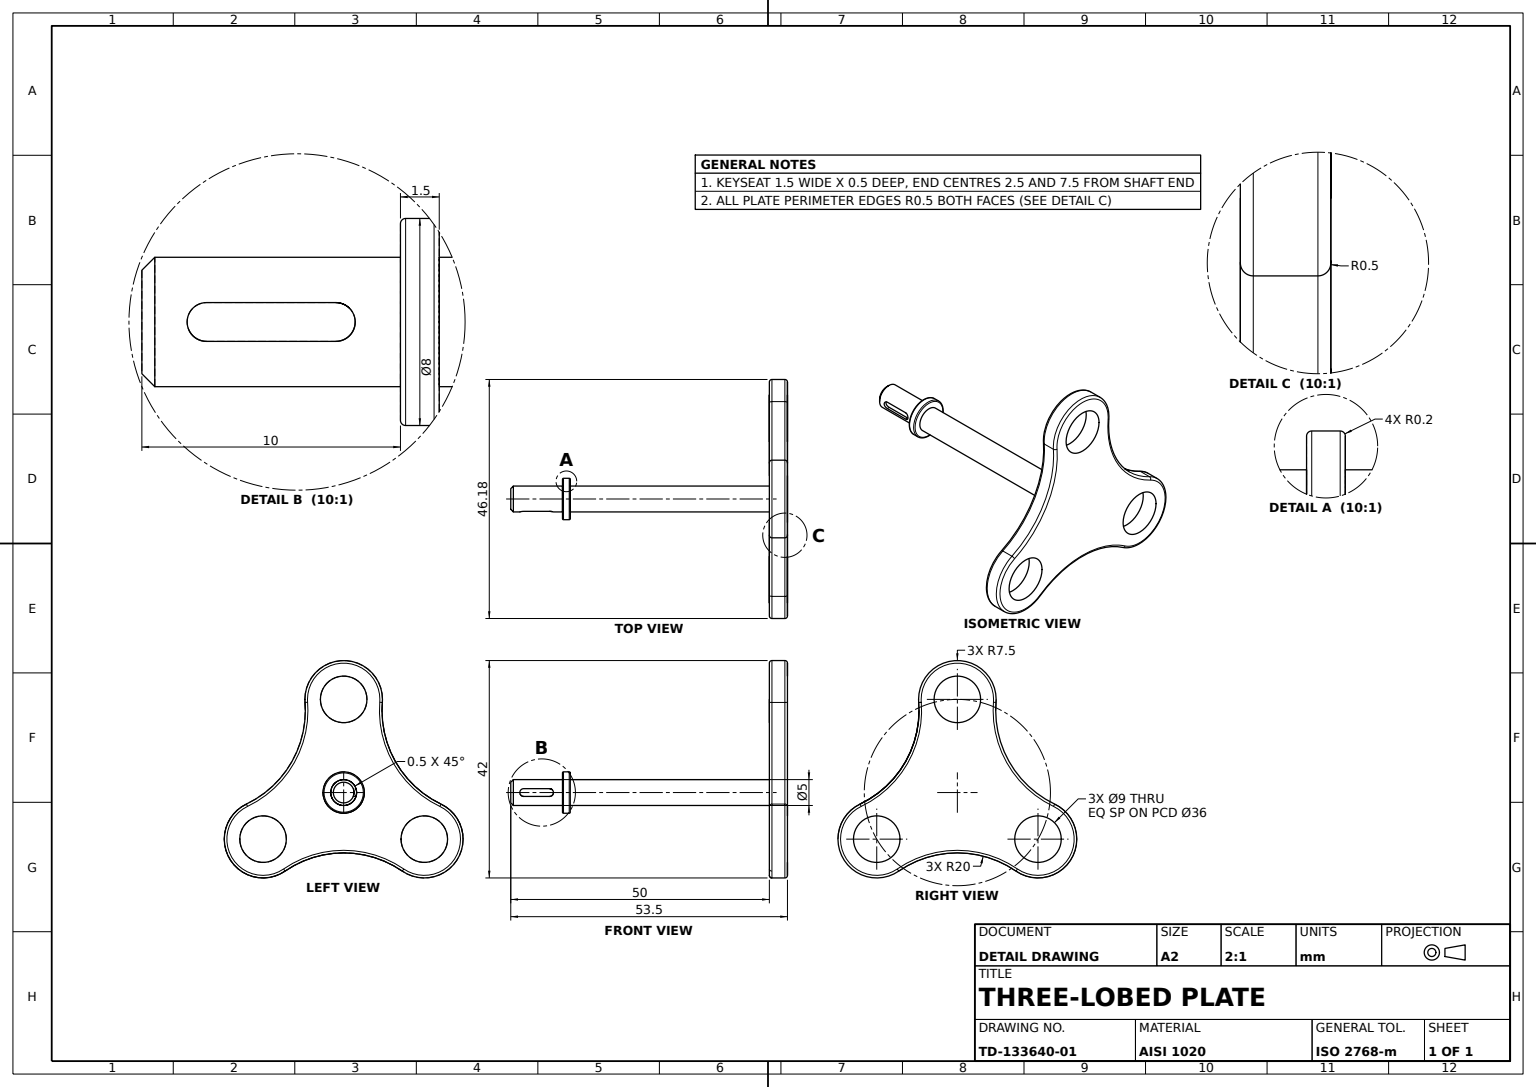
SolidWorks part; units mm, degrees
material "AISI 1020"
ref_plane "Front Plane" through (0, 0, 0) normal (0, 0, 1) x (1, 0, 0)
ref_plane "Top Plane" through (0, 0, 0) normal (0, 1, 0) x (1, 0, 0)
ref_plane "Right Plane" through (0, 0, 0) normal (1, 0, 0) x (0, 0, -1)
sketch "Carrier Plate Profile" plane through (0, 0, 0) normal (0, 0, 1) x (1, 0, 0)
  circle A0 centre (0, 18) radius 7.5
  circle A1 centre (0, 18) radius 4.5
  circle A2 centre (15.5885, -9) radius 7.5
  circle A3 centre (15.5885, -9) radius 4.5
  circle A4 centre (-15.5885, -9) radius 7.5
  circle A5 centre (-15.5885, -9) radius 4.5
  arc A6 (7.4766, 17.4075) -> (18.8136, -2.2289) centre (27.4141, 15.8275) ccw
  arc A7 (11.3371, -15.1786) -> (-11.3371, -15.1786) centre (0, -31.655) ccw
  arc A8 (-18.8136, -2.2289) -> (-7.4766, 17.4075) centre (-27.4141, 15.8275) ccw
  point P12 (0, 0)
  point P22 (0, 0)
  dimension "D1" = 15
  dimension "D2" = 9
  dimension "D5" = 20
  dimension "D3" = 18
  dimension "D4" = 3
  dimension "D6" = 3
extrude "Carrier Plate" add sketch "Carrier Plate Profile" along normal blind 3.5 contours A2 A3 | A0 A1 | A4 A5 | A8 A4 A7 A2 A6 A0
sketch "Shaft Profile Ø5" plane through (0, 0, 3.5) normal (0, 0, 1) x (1, 0, 0)
  circle A0 centre (0, 0) radius 2.5
  dimension "D1" = 5
extrude "Shaft Ø5x50" add sketch "Shaft Profile Ø5" along normal blind 50
sketch "Collar Profile" plane through (0, 0, 53.5) normal (0, 0, 1) x (1, 0, 0)
  circle A0 centre (0, 0) radius 4
  dimension "D1" = 8
extrude "Shaft Collar" add sketch "Collar Profile" against normal blind 1.5 from offset 10 offset against normal yes
sketch "Keyseat Profile" plane through (0, 0, 0) normal (1, 0, 0) x (0, 0, -1)
  line L0 (-51, 0) -> (-46, 0) construction
  line L1 (-51, 0.75) -> (-46, 0.75)
  line L2 (-51, -0.75) -> (-46, -0.75)
  line L3 (-53.5, 2.5) -> (-53.5, -2.5) construction
  arc A0 (-51, 0.75) -> (-51, -0.75) centre (-51, 0) ccw
  arc A1 (-46, -0.75) -> (-46, 0.75) centre (-46, 0) ccw
  point P2 (-48.5, 0)
  dimension "D1" = 5
  dimension "D2" = 5
  dimension "D3" = 1.5
extrude "Shaft Keyseat" cut sketch "Keyseat Profile" against normal offset from surface (3.146 mm away) 0.5 from offset 5
chamfer "Shaft End Chamfer" distance 0.5 angle 45 1 edges at (2.5, 0, 53.5)
fillet "Collar Edge Fillet" radius 0.2 2 edges at (4, 0, 43.5) (4, 0, 42)
fillet "Plate Edge Fillet" radius 0.5 12 edges at (0, 25.5, 0) (0, 25.5, 3.5) (-10.0935, 5.8275, 0) (-10.0935, 5.8275, 3.5) (-22.0836, -12.75, 0) (-22.0836, -12.75, 3.5) (0, -11.655, 0) (0, -11.655, 3.5) (22.0836, -12.75, 0) (22.0836, -12.75, 3.5) (10.0935, 5.8275, 0) (10.0935, 5.8275, 3.5)
